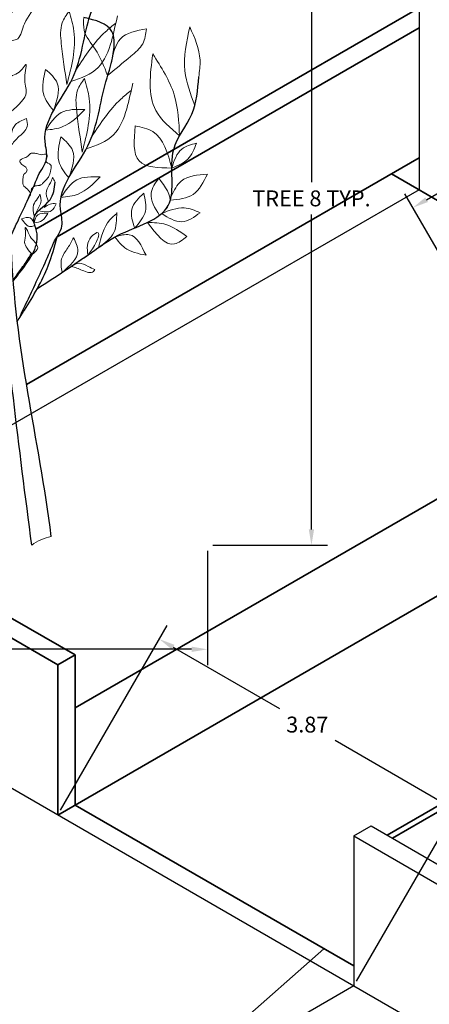
# Model space of a CAD drawing. Units: metres. Extents: x 12735 to 25554, y 20954 to 41989.
# Tile 3 of 15: x 12743.97 to 12748.61, y 20963.53 to 20974.68. Entities that reach past the tile are written whole.
import ezdxf

# ---------------------------------------------------------------- set-up
doc = ezdxf.new("R2010")
doc.units = ezdxf.units.M
doc.layers.get('Defpoints').update_dxf_attribs({"lineweight": 13})
for name, color, linetype, lineweight in [('A-ANNO-DIMS', 2, 'Continuous', 18), ('A-ELEV', 7, 'Continuous', 35), ('C-SITE', 8, 'Continuous', 25), ('TREES', 72, 'Continuous', 18)]:
    doc.layers.add(name, color=color, linetype=linetype, lineweight=lineweight)
doc.layers.add('STEM', color=32, linetype='Continuous')
doc.styles.get("Standard").update_dxf_attribs({"font": 'arial.ttf'})
doc.dimstyles.get("Standard").update_dxf_attribs({"dimtxt": 0.18, "dimasz": 0.18, "dimexe": 0.18, "dimexo": 0.0625, "dimgap": 0.09, "dimtad": 0, "dimtih": 1, "dimtoh": 1, "dimdec": 4, "dimzin": 0, "dimdsep": 46, "dimtxsty": 'Standard', "dimcen": 0.09, "dimadec": 0, "dimazin": 0, "dimtfac": 1, "dimtdec": 4, "dimtofl": 0, "dimtmove": 0, "dimatfit": 3, "dimfxl": 1, "dimtolj": 1, "dimtzin": 0, "dimarcsym": 0})

# ---------------------------------------------------------------- blocks, each defined once
blk = doc.blocks.new('TREES')
blk.add_line((12743.7, 20972.648), (12743.7, 20972.648))
at = {"layer": 'STEM'}
for points, knots in [([(12743.791, 20972.546), (12743.793, 20972.564), (12743.795, 20972.582), (12743.797, 20972.6), (12743.801, 20972.637), (12743.806, 20972.674), (12743.81, 20972.711), (12743.845, 20973.018), (12743.938, 20973.826), (12743.743, 20974.806), (12743.607, 20975.634), (12743.413, 20975.893), (12743.333, 20975.999)], [-0.164913, -0.164913, -0.164913, -0.164913, -0.110972, -0.110972, -0.110972, 0, 0, 0, 0.920963, 2.426088, 2.990404, 3.384799, 3.384799, 3.384799, 3.384799]), ([(12743.7, 20972.648), (12743.691, 20972.807), (12743.671, 20973.194), (12743.257, 20973.699), (12743.111, 20974.379), (12743.038, 20974.998), (12742.993, 20975.377), (12742.974, 20975.54)], [0, 0, 0, 0, 0.469346, 1.137622, 1.869488, 2.521439, 3.013071, 3.013071, 3.013071, 3.013071]), ([(12743.874, 20972.227), (12743.898, 20972.277), (12743.921, 20972.328), (12743.945, 20972.378), (12744.022, 20972.541), (12744.105, 20972.717), (12744.205, 20972.963), (12744.312, 20973.088), (12744.183, 20973.501), (12744.667, 20973.973), (12744.707, 20974.64), (12744.896, 20975.012), (12744.823, 20975.434), (12744.85, 20975.23), (12744.867, 20975.1)], [-0.166951, -0.166951, -0.166951, -0.166951, 0, 0, 0, 0.539768, 0.582066, 0.798222, 0.98781, 1.7696, 2.524754, 2.899414, 3.105113, 3.460848, 3.460848, 3.460848, 3.460848]), ([(12743.728, 20972.218), (12743.63, 20972.372), (12743.383, 20972.76), (12742.753, 20973.07), (12742.291, 20973.419), (12741.984, 20973.759), (12741.959, 20974.098), (12741.675, 20974.346), (12741.563, 20974.543), (12741.494, 20974.663)], [0, 0, 0, 0, 0.542161, 1.359078, 2.03444, 2.290187, 2.703676, 2.968549, 3.382864, 3.382864, 3.382864, 3.382864]), ([(12743.967, 20971.294), (12743.987, 20971.335), (12744.006, 20971.376), (12744.026, 20971.417), (12744.057, 20971.483), (12744.088, 20971.549), (12744.119, 20971.615), (12744.196, 20971.778), (12744.279, 20971.954), (12744.378, 20972.2), (12744.486, 20972.325), (12744.357, 20972.738), (12744.836, 20973.215), (12744.895, 20973.862), (12745.051, 20974.269), (12745.045, 20974.62), (12744.834, 20974.67), (12744.7, 20974.701)], [-0.355099, -0.355099, -0.355099, -0.355099, -0.218492, -0.218492, -0.218492, 0, 0, 0, 0.539768, 0.582066, 0.798222, 0.98781, 1.7696, 2.524754, 2.899414, 3.105113, 3.460848, 3.460848, 3.460848, 3.460848]), ([(12744.175, 20971.633), (12744.383, 20971.767), (12744.692, 20971.967), (12745.149, 20972.305), (12745.828, 20972.463), (12745.606, 20973.185), (12745.967, 20973.583), (12745.99, 20973.882), (12746.002, 20974.029)], [0, 0, 0, 0, 0.736164, 1.094646, 1.754618, 2.392389, 2.840214, 3.27091, 3.27091, 3.27091, 3.27091]), ([(12743.381, 20973.588), (12743.52, 20973.4), (12743.728, 20973.118), (12743.725, 20972.776), (12743.724, 20972.661), (12743.724, 20972.661), (12743.724, 20972.661), (12743.724, 20972.661), (12743.724, 20972.65), (12743.724, 20972.639), (12743.724, 20972.627)], [0, 0, 0, 0, 0.673099, 1.009429, 1.009429, 1.009429, 1.009429, 1.009429, 1.009429, 1.043412, 1.043412, 1.043412, 1.043412]), ([(12743.814, 20972.505), (12743.817, 20972.531), (12743.819, 20972.556), (12743.822, 20972.581), (12743.827, 20972.63), (12743.832, 20972.679), (12743.838, 20972.727), (12743.847, 20972.813), (12743.865, 20972.982), (12743.864, 20973.152), (12743.864, 20973.236)], [-0.2227932, -0.2227932, -0.2227932, -0.2227932, -0.1464713, -0.1464713, -0.1464713, 0, 0, 0, 0.2578951, 0.5103882, 0.5103882, 0.5103882, 0.5103882]), ([(12743.902, 20971.717), (12743.93, 20971.754), (12743.959, 20971.791), (12743.988, 20971.829), (12743.988, 20971.829), (12743.988, 20971.829), (12743.988, 20971.829), (12744.096, 20971.973), (12744.236, 20972.16), (12744.082, 20972.476), (12744.347, 20972.598), (12744.368, 20972.766), (12744.376, 20972.837)], [-0.129757, -0.129757, -0.129757, -0.129757, 0, 0, 0, 0, 0, 0, 0.485118, 0.62751, 0.913144, 1.120766, 1.120766, 1.120766, 1.120766]), ([(12744.111, 20968.725), (12743.967, 20969.837), (12743.799, 20971.142), (12743.712, 20972.453), (12743.7, 20972.648)], [0, 0, 0, 0, 3.359203, 3.944548, 3.944548, 3.944548, 3.944548]), ([(12744.332, 20968.825), (12744.189, 20969.936), (12743.871, 20971.161), (12743.872, 20972.51), (12743.7, 20972.648)], [0, 0, 0, 0, 3.359203, 3.972384, 3.972384, 3.972384, 3.972384]), ([(12743.597, 20972.418), (12743.533, 20972.41), (12743.292, 20972.379), (12742.889, 20972.351), (12742.364, 20972.241), (12741.803, 20972.489), (12741.157, 20972.302), (12740.698, 20972.258), (12740.474, 20972.237)], [0, 0, 0, 0, 0.193148, 0.727923, 1.218416, 1.762371, 2.471743, 3.152626, 3.152626, 3.152626, 3.152626]), ([(12743.181, 20972.372), (12743.296, 20972.37), (12743.441, 20972.368), (12743.583, 20972.39), (12743.613, 20972.395)], [0, 0, 0, 0, 0.3435042, 0.4329772, 0.4329772, 0.4329772, 0.4329772]), ([(12743.948, 20971.264), (12743.975, 20971.305), (12744.002, 20971.345), (12744.029, 20971.386), (12744.029, 20971.386), (12744.029, 20971.386), (12744.029, 20971.386), (12744.129, 20971.55), (12744.289, 20971.812), (12744.368, 20972.107), (12744.398, 20972.218)], [-0.148605, -0.148605, -0.148605, -0.148605, 0, 0, 0, 0, 0, 0, 0.572176, 0.914425, 0.914425, 0.914425, 0.914425]), ([(12743.901, 20971.729), (12743.929, 20971.768), (12743.958, 20971.808), (12743.986, 20971.847), (12743.986, 20971.847), (12743.986, 20971.847), (12743.986, 20971.847), (12744.02, 20971.892), (12744.062, 20971.951), (12744.099, 20972.014), (12744.107, 20972.028)], [-0.1467707, -0.1467707, -0.1467707, -0.1467707, 0, 0, 0, 0, 0, 0, 0.1684242, 0.2179474, 0.2179474, 0.2179474, 0.2179474]), ([(12743.81, 20971.258), (12743.646, 20971.316), (12743.283, 20971.443), (12742.486, 20971.453), (12741.888, 20971.61), (12741.494, 20971.714)], [0, 0, 0, 0, 0.519056, 1.146346, 2.366016, 2.366016, 2.366016, 2.366016])]:
    blk.add_open_spline(points, degree=3, knots=knots, dxfattribs=at)
blk.add_open_spline([(12744.644, 20971.941), (12744.672, 20971.961), (12744.701, 20971.98), (12744.73, 20972)], degree=3, dxfattribs=at)
at = {"layer": 'TREES'}
for points, knots in [([(12743.584, 20975.586), (12743.37, 20975.718), (12743.075, 20975.9), (12743.022, 20976.725), (12743.333, 20976.097), (12743.574, 20975.612)], [0, 0, 0, 0, 0.724771, 1.002271, 1.932196, 1.932196, 1.932196, 1.932196]), ([(12743.021, 20975.14), (12743.019, 20975.277), (12743.016, 20975.483), (12742.921, 20975.662), (12742.889, 20975.721)], [0, 0, 0, 0, 0.4023849, 0.6031293, 0.6031293, 0.6031293, 0.6031293]), ([(12743.021, 20975.14), (12742.985, 20975.224), (12742.928, 20975.356), (12742.766, 20975.539), (12742.854, 20975.638), (12742.901, 20975.69)], [0, 0, 0, 0, 0.2845416, 0.4465287, 0.6279758, 0.6279758, 0.6279758, 0.6279758]), ([(12743.718, 20974.979), (12743.671, 20975.164), (12743.598, 20975.454), (12743.323, 20975.534), (12743.223, 20975.563)], [0, 0, 0, 0, 0.519429, 0.8155501, 0.8155501, 0.8155501, 0.8155501]), ([(12743.223, 20975.563), (12743.266, 20975.448), (12743.36, 20975.195), (12743.592, 20975.055), (12743.718, 20974.979)], [0, 0, 0, 0, 0.3595778, 0.7860105, 0.7860105, 0.7860105, 0.7860105]), ([(12743.737, 20974.871), (12743.729, 20975.055), (12743.718, 20975.333), (12743.914, 20975.516), (12743.981, 20975.578)], [0, 0, 0, 0, 0.5134638, 0.7779111, 0.7779111, 0.7779111, 0.7779111]), ([(12743.737, 20974.871), (12743.801, 20974.971), (12743.939, 20975.186), (12743.966, 20975.441), (12743.981, 20975.578)], [0, 0, 0, 0, 0.351068, 0.7565079, 0.7565079, 0.7565079, 0.7565079]), ([(12741.648, 20974.411), (12741.519, 20974.547), (12741.281, 20974.798), (12741.642, 20974.995), (12741.673, 20975.511), (12741.684, 20975.149), (12741.787, 20975.033), (12741.768, 20974.824), (12741.781, 20974.575), (12741.641, 20974.411), (12741.569, 20974.326)], [0, 0, 0, 0, 0.446457, 0.821839, 1.096823, 1.294203, 1.491123, 1.594729, 1.894892, 2.216107, 2.216107, 2.216107, 2.216107]), ([(12743.031, 20975.058), (12743.048, 20975.139), (12743.077, 20975.281), (12743.184, 20975.377), (12743.231, 20975.418)], [0, 0, 0, 0, 0.2398723, 0.4207027, 0.4207027, 0.4207027, 0.4207027]), ([(12743.037, 20975.007), (12743.075, 20975.058), (12743.166, 20975.181), (12743.207, 20975.33), (12743.231, 20975.418)], [0, 0, 0, 0, 0.1895117, 0.457602, 0.457602, 0.457602, 0.457602]), ([(12744.796, 20974.806), (12744.757, 20974.909), (12744.688, 20975.088), (12744.514, 20975.28), (12744.523, 20975.414), (12744.526, 20975.464)], [0, 0, 0, 0, 0.3323117, 0.5782809, 0.7232611, 0.7232611, 0.7232611, 0.7232611]), ([(12744.805, 20974.813), (12744.804, 20974.918), (12744.803, 20975.076), (12744.822, 20975.37), (12744.643, 20975.427), (12744.526, 20975.464)], [0, 0, 0, 0, 0.3224266, 0.4885617, 0.8037384, 0.8037384, 0.8037384, 0.8037384]), ([(12743.07, 20974.733), (12742.98, 20974.863), (12742.848, 20975.053), (12742.433, 20975.446), (12742.649, 20974.915), (12742.651, 20974.573), (12742.961, 20974.576), (12743.034, 20974.678), (12743.071, 20974.73)], [0, 0, 0, 0, 0.54832, 0.799685, 1.166614, 1.565159, 1.742127, 1.925713, 1.925713, 1.925713, 1.925713]), ([(12744.796, 20974.806), (12744.882, 20974.878), (12745.017, 20974.992), (12745.211, 20975.15), (12745.228, 20975.277), (12745.236, 20975.337)], [0, 0, 0, 0, 0.3416822, 0.5370609, 0.7122352, 0.7122352, 0.7122352, 0.7122352]), ([(12744.839, 20974.951), (12744.859, 20975.055), (12744.903, 20975.272), (12745.122, 20975.315), (12745.236, 20975.337)], [0, 0, 0, 0, 0.2913456, 0.6064398, 0.6064398, 0.6064398, 0.6064398]), ([(12743.814, 20974.4), (12743.798, 20974.494), (12743.764, 20974.693), (12744.115, 20975.006), (12744.156, 20974.79), (12744.01, 20974.677), (12743.989, 20974.434), (12743.864, 20974.438), (12743.809, 20974.439)], [0, 0, 0, 0, 0.311146, 0.650746, 0.669061, 0.940573, 1.125337, 1.270427, 1.270427, 1.270427, 1.270427]), ([(12743.191, 20974.047), (12743.14, 20974.139), (12743.026, 20974.346), (12743.367, 20974.877), (12743.354, 20974.597), (12743.309, 20974.413), (12743.358, 20974.125), (12743.218, 20974.059), (12743.191, 20974.047)], [0, 0, 0, 0, 0.337622, 0.758697, 0.837919, 1.040495, 1.406258, 1.489574, 1.489574, 1.489574, 1.489574]), ([(12742.028, 20973.754), (12742.003, 20973.912), (12741.953, 20974.218), (12742.174, 20974.414), (12742.283, 20974.81), (12742.258, 20974.48), (12742.304, 20974.323), (12742.246, 20974.069), (12742.227, 20973.932), (12742.006, 20973.671), (12742.066, 20973.72), (12742.075, 20973.727)], [0, 0, 0, 0, 0.436736, 0.842969, 1.012738, 1.21393, 1.403734, 1.613178, 1.897283, 2.067562, 2.097274, 2.097274, 2.097274, 2.097274]), ([(12744.509, 20973.941), (12744.486, 20974.093), (12744.451, 20974.322), (12744.425, 20974.623), (12744.504, 20974.731), (12744.534, 20974.773)], [0, 0, 0, 0, 0.4681587, 0.7056034, 0.8580265, 0.8580265, 0.8580265, 0.8580265]), ([(12744.534, 20974.773), (12744.556, 20974.698), (12744.634, 20974.425), (12744.562, 20974.144), (12744.509, 20973.941)], [0, 0, 0, 0, 0.2327329, 0.8431329, 0.8431329, 0.8431329, 0.8431329]), ([(12744.554, 20973.975), (12744.669, 20974.016), (12744.893, 20974.094), (12745.019, 20974.421), (12745.06, 20974.624), (12745.08, 20974.72)], [0, 0, 0, 0, 0.348929, 0.678298, 0.9763146, 0.9763146, 0.9763146, 0.9763146]), ([(12743.835, 20974.249), (12743.789, 20974.346), (12743.724, 20974.484), (12743.556, 20974.594), (12743.468, 20974.601), (12743.424, 20974.604)], [0, 0, 0, 0, 0.3158223, 0.4463774, 0.5774617, 0.5774617, 0.5774617, 0.5774617]), ([(12743.424, 20974.604), (12743.442, 20974.527), (12743.487, 20974.324), (12743.715, 20974.191), (12743.841, 20974.206), (12743.841, 20974.206)], [0, 0, 0, 0, 0.2361186, 0.6165307, 0.6167763, 0.6167763, 0.6167763, 0.6167763]), ([(12744.618, 20974.118), (12744.717, 20974.268), (12744.844, 20974.462), (12745.022, 20974.606), (12745.062, 20974.638)], [0, 0, 0, 0, 0.5333846, 0.686651, 0.686651, 0.686651, 0.686651]), ([(12744.97, 20974.043), (12744.931, 20974.146), (12744.862, 20974.325), (12744.688, 20974.517), (12744.697, 20974.651), (12744.7, 20974.701)], [0, 0, 0, 0, 0.3323117, 0.5782809, 0.7232611, 0.7232611, 0.7232611, 0.7232611]), ([(12745.957, 20973.706), (12745.908, 20973.835), (12745.798, 20974.123), (12745.864, 20974.427), (12745.9, 20974.594)], [0, 0, 0, 0, 0.4051126, 0.906838, 0.906838, 0.906838, 0.906838]), ([(12745.9, 20974.594), (12745.955, 20974.471), (12746.037, 20974.287), (12746.01, 20974.092), (12746.002, 20974.029)], [0, 0, 0, 0, 0.3943838, 0.5836156, 0.5836156, 0.5836156, 0.5836156]), ([(12744.97, 20974.043), (12745.056, 20974.115), (12745.191, 20974.229), (12745.385, 20974.387), (12745.402, 20974.514), (12745.41, 20974.574)], [0, 0, 0, 0, 0.3416822, 0.5370609, 0.7122352, 0.7122352, 0.7122352, 0.7122352]), ([(12745.013, 20974.188), (12745.033, 20974.292), (12745.077, 20974.509), (12745.296, 20974.552), (12745.41, 20974.574)], [0, 0, 0, 0, 0.2913456, 0.6064398, 0.6064398, 0.6064398, 0.6064398]), ([(12743.128, 20974.182), (12743.019, 20974.275), (12742.841, 20974.427), (12742.65, 20974.313), (12742.577, 20974.27)], [0, 0, 0, 0, 0.3785086, 0.6144536, 0.6144536, 0.6144536, 0.6144536]), ([(12742.577, 20974.27), (12742.635, 20974.174), (12742.755, 20973.977), (12743.187, 20974.003), (12743.173, 20974.131), (12743.172, 20974.137)], [0, 0, 0, 0, 0.3386751, 0.6999446, 0.7185805, 0.7185805, 0.7185805, 0.7185805]), ([(12745.785, 20973.361), (12745.68, 20973.449), (12745.404, 20973.684), (12745.451, 20974.057), (12745.481, 20974.288)], [0, 0, 0, 0, 0.391493, 1.034106, 1.034106, 1.034106, 1.034106]), ([(12745.481, 20974.288), (12745.577, 20974.138), (12745.76, 20973.855), (12745.777, 20973.519), (12745.785, 20973.361)], [0, 0, 0, 0, 0.5245256, 0.9915723, 0.9915723, 0.9915723, 0.9915723]), ([(12741.943, 20974.016), (12741.835, 20974.13), (12741.594, 20974.382), (12741.272, 20973.991), (12740.687, 20974.27), (12741.289, 20973.836), (12741.63, 20973.742), (12741.878, 20973.799), (12742.016, 20973.831)], [0, 0, 0, 0, 0.397812, 0.88569, 1.156328, 1.66735, 1.991498, 2.394837, 2.394837, 2.394837, 2.394837]), ([(12743.879, 20973.555), (12743.816, 20973.752), (12743.731, 20974.021), (12743.982, 20974.067), (12744.068, 20974.224), (12744.006, 20973.984), (12744.093, 20973.824), (12743.961, 20973.709), (12743.879, 20973.638)], [0, 0, 0, 0, 0.469961, 0.638827, 0.705595, 0.853148, 1.022788, 1.296962, 1.296962, 1.296962, 1.296962]), ([(12744.356, 20973.647), (12744.309, 20973.708), (12744.202, 20973.846), (12744.245, 20974.018), (12744.268, 20974.113)], [0, 0, 0, 0, 0.2209277, 0.4981889, 0.4981889, 0.4981889, 0.4981889]), ([(12744.268, 20974.113), (12744.323, 20974.065), (12744.46, 20973.94), (12744.395, 20973.758), (12744.356, 20973.647)], [0, 0, 0, 0, 0.203616, 0.5174389, 0.5174389, 0.5174389, 0.5174389]), ([(12742.389, 20973.356), (12742.341, 20973.437), (12742.234, 20973.617), (12742.458, 20973.799), (12742.48, 20973.946), (12742.486, 20973.991)], [0, 0, 0, 0, 0.251735, 0.5591808, 0.6938707, 0.6938707, 0.6938707, 0.6938707]), ([(12742.486, 20973.991), (12742.542, 20973.959), (12742.68, 20973.88), (12742.598, 20973.572), (12742.464, 20973.433), (12742.389, 20973.356)], [0, 0, 0, 0, 0.1746142, 0.4385715, 0.7703441, 0.7703441, 0.7703441, 0.7703441]), ([(12743.381, 20973.588), (12743.369, 20973.67), (12743.344, 20973.833), (12743.453, 20973.958), (12743.508, 20974.02)], [0, 0, 0, 0, 0.2360196, 0.4713289, 0.4713289, 0.4713289, 0.4713289]), ([(12743.381, 20973.588), (12743.434, 20973.649), (12743.541, 20973.774), (12743.519, 20973.937), (12743.508, 20974.02)], [0, 0, 0, 0, 0.2309694, 0.4699481, 0.4699481, 0.4699481, 0.4699481]), ([(12744.683, 20973.178), (12744.66, 20973.33), (12744.625, 20973.559), (12744.599, 20973.86), (12744.677, 20973.968), (12744.708, 20974.01)], [0, 0, 0, 0, 0.4681587, 0.7056034, 0.8580265, 0.8580265, 0.8580265, 0.8580265]), ([(12744.708, 20974.01), (12744.73, 20973.935), (12744.807, 20973.662), (12744.735, 20973.381), (12744.683, 20973.178)], [0, 0, 0, 0, 0.2327329, 0.8431329, 0.8431329, 0.8431329, 0.8431329]), ([(12744.728, 20973.213), (12744.843, 20973.253), (12745.067, 20973.331), (12745.193, 20973.658), (12745.234, 20973.861), (12745.254, 20973.957)], [0, 0, 0, 0, 0.348929, 0.678298, 0.9763146, 0.9763146, 0.9763146, 0.9763146]), ([(12743.851, 20973.09), (12743.747, 20973.196), (12743.578, 20973.368), (12743.647, 20973.644), (12743.671, 20973.769), (12743.679, 20973.81)], [0, 0, 0, 0, 0.4076044, 0.6640272, 0.7921335, 0.7921335, 0.7921335, 0.7921335]), ([(12743.679, 20973.81), (12743.708, 20973.778), (12743.776, 20973.703), (12743.798, 20973.443), (12743.829, 20973.238), (12743.851, 20973.09)], [0, 0, 0, 0, 0.125659, 0.2981213, 0.7527794, 0.7527794, 0.7527794, 0.7527794]), ([(12744.792, 20973.355), (12744.891, 20973.505), (12745.018, 20973.699), (12745.196, 20973.843), (12745.236, 20973.876)], [0, 0, 0, 0, 0.5333846, 0.686651, 0.686651, 0.686651, 0.686651]), ([(12743.364, 20973.617), (12743.288, 20973.661), (12743.124, 20973.754), (12742.939, 20973.715), (12742.84, 20973.694)], [0, 0, 0, 0, 0.2535199, 0.5460217, 0.5460217, 0.5460217, 0.5460217]), ([(12742.221, 20973.506), (12741.989, 20973.602), (12741.674, 20973.731), (12741.536, 20973.471), (12741.5, 20973.404)], [0, 0, 0, 0, 0.6060397, 0.8197481, 0.8197481, 0.8197481, 0.8197481]), ([(12743.253, 20972.784), (12743.147, 20972.854), (12742.919, 20973.005), (12742.8, 20973.728), (12742.973, 20973.491), (12743.022, 20973.422)], [0, 0, 0, 0, 0.420416, 0.90702, 1.103207, 1.103207, 1.103207, 1.103207]), ([(12742.84, 20973.694), (12742.956, 20973.634), (12743.128, 20973.545), (12743.306, 20973.6), (12743.364, 20973.617)], [0, 0, 0, 0, 0.369417, 0.546183, 0.546183, 0.546183, 0.546183]), ([(12744.268, 20973.425), (12744.32, 20973.505), (12744.424, 20973.666), (12744.615, 20973.662), (12744.711, 20973.66)], [0, 0, 0, 0, 0.2669279, 0.5349854, 0.5349854, 0.5349854, 0.5349854]), ([(12744.268, 20973.425), (12744.336, 20973.433), (12744.51, 20973.454), (12744.635, 20973.582), (12744.711, 20973.66)], [0, 0, 0, 0, 0.1990667, 0.5143408, 0.5143408, 0.5143408, 0.5143408]), ([(12741.493, 20973.429), (12741.634, 20973.396), (12741.906, 20973.333), (12742.16, 20973.449), (12742.283, 20973.505)], [0, 0, 0, 0, 0.420024, 0.8136231, 0.8136231, 0.8136231, 0.8136231]), ([(12743.864, 20973.236), (12743.891, 20973.272), (12743.952, 20973.35), (12744.077, 20973.438), (12744.058, 20973.527), (12744.051, 20973.558)], [0, 0, 0, 0, 0.1377377, 0.3031534, 0.3935537, 0.3935537, 0.3935537, 0.3935537]), ([(12743.866, 20973.267), (12743.872, 20973.352), (12743.881, 20973.49), (12744.004, 20973.539), (12744.051, 20973.558)], [0, 0, 0, 0, 0.2295676, 0.3730638, 0.3730638, 0.3730638, 0.3730638]), ([(12743.022, 20973.422), (12743.059, 20973.426), (12743.334, 20973.456), (12743.256, 20972.956), (12743.349, 20972.723), (12743.36, 20972.696)], [0, 0, 0, 0, 0.1039343, 0.7792863, 0.8705393, 0.8705393, 0.8705393, 0.8705393]), ([(12745.697, 20972.996), (12745.547, 20972.999), (12745.238, 20973.004), (12745.268, 20973.314), (12745.283, 20973.473)], [0, 0, 0, 0, 0.3799868, 0.779071, 0.779071, 0.779071, 0.779071]), ([(12745.283, 20973.473), (12745.354, 20973.458), (12745.585, 20973.409), (12745.651, 20973.165), (12745.697, 20972.996)], [0, 0, 0, 0, 0.2074949, 0.6743984, 0.6743984, 0.6743984, 0.6743984]), ([(12741.595, 20972.406), (12741.523, 20972.496), (12741.318, 20972.752), (12741.336, 20973.087), (12741.348, 20973.304)], [0, 0, 0, 0, 0.3390919, 0.9589007, 0.9589007, 0.9589007, 0.9589007]), ([(12741.348, 20973.304), (12741.406, 20973.227), (12741.6, 20972.969), (12741.591, 20972.637), (12741.585, 20972.405)], [0, 0, 0, 0, 0.2865181, 0.9509807, 0.9509807, 0.9509807, 0.9509807]), ([(12743.621, 20973.151), (12743.561, 20973.233), (12743.473, 20973.354), (12743.333, 20973.334), (12743.288, 20973.327)], [0, 0, 0, 0, 0.2726158, 0.4022356, 0.4022356, 0.4022356, 0.4022356]), ([(12743.288, 20973.327), (12743.325, 20973.265), (12743.399, 20973.138), (12743.546, 20973.147), (12743.621, 20973.151)], [0, 0, 0, 0, 0.199886, 0.4070645, 0.4070645, 0.4070645, 0.4070645]), ([(12744.53, 20972.884), (12744.482, 20972.945), (12744.376, 20973.084), (12744.419, 20973.255), (12744.442, 20973.351)], [0, 0, 0, 0, 0.2209277, 0.4981889, 0.4981889, 0.4981889, 0.4981889]), ([(12744.442, 20973.351), (12744.496, 20973.302), (12744.634, 20973.177), (12744.569, 20972.995), (12744.53, 20972.884)], [0, 0, 0, 0, 0.203616, 0.5174389, 0.5174389, 0.5174389, 0.5174389]), ([(12745.697, 20972.996), (12745.724, 20973.08), (12745.77, 20973.226), (12745.915, 20973.262), (12745.976, 20973.277)], [0, 0, 0, 0, 0.2439478, 0.4222058, 0.4222058, 0.4222058, 0.4222058]), ([(12745.697, 20972.996), (12745.764, 20973.024), (12745.897, 20973.078), (12745.95, 20973.211), (12745.976, 20973.277)], [0, 0, 0, 0, 0.2073861, 0.4117039, 0.4117039, 0.4117039, 0.4117039]), ([(12744.074, 20972.655), (12744.086, 20972.673), (12744.124, 20972.731), (12743.998, 20972.782), (12744.014, 20972.867), (12744.011, 20972.925), (12744.052, 20972.944), (12744.07, 20973.015), (12743.988, 20973.027), (12743.97, 20973.091), (12744.03, 20973.11), (12744.072, 20973.132), (12744.097, 20973.169), (12744.133, 20973.163), (12744.172, 20973.164), (12744.216, 20973.136), (12744.296, 20973.17), (12744.282, 20973.105), (12744.259, 20973.057), (12744.341, 20973.048), (12744.328, 20972.986), (12744.32, 20972.935), (12744.299, 20972.884), (12744.258, 20972.852), (12744.236, 20972.821), (12744.215, 20972.805), (12744.179, 20972.793), (12744.139, 20972.807), (12744.095, 20972.746), (12744.111, 20972.739), (12744.111, 20972.739)], [0, 0, 0, 0, 0.055886, 0.185472, 0.25227, 0.305988, 0.338368, 0.378405, 0.48523, 0.4997, 0.565031, 0.618654, 0.656012, 0.680602, 0.71942, 0.77395, 0.836088, 0.890088, 0.913694, 0.979696, 1.032481, 1.0683, 1.142133, 1.186825, 1.224162, 1.25438, 1.26551, 1.333296, 1.383591, 1.385324, 1.385324, 1.385324, 1.385324]), ([(12742.983, 20972.961), (12742.799, 20973.009), (12742.463, 20973.098), (12742.071, 20972.928), (12741.893, 20972.798), (12741.839, 20972.759)], [0, 0, 0, 0, 0.553894, 1.01265, 1.215779, 1.215779, 1.215779, 1.215779]), ([(12743.669, 20972.977), (12743.606, 20973.025), (12743.504, 20973.102), (12743.398, 20973.043), (12743.358, 20973.021)], [0, 0, 0, 0, 0.2119595, 0.340544, 0.340544, 0.340544, 0.340544]), ([(12741.839, 20972.759), (12741.949, 20972.7), (12742.323, 20972.501), (12742.684, 20972.786), (12742.939, 20972.987)], [0, 0, 0, 0, 0.355589, 1.206871, 1.206871, 1.206871, 1.206871]), ([(12743.358, 20973.021), (12743.426, 20972.983), (12743.527, 20972.926), (12743.633, 20972.964), (12743.669, 20972.977)], [0, 0, 0, 0, 0.2166399, 0.3265492, 0.3265492, 0.3265492, 0.3265492]), ([(12745.681, 20972.634), (12745.776, 20972.643), (12745.97, 20972.661), (12746.056, 20972.838), (12746.1, 20972.929)], [0, 0, 0, 0, 0.2646598, 0.5464061, 0.5464061, 0.5464061, 0.5464061]), ([(12745.691, 20972.679), (12745.723, 20972.743), (12745.803, 20972.904), (12745.989, 20972.919), (12746.1, 20972.929)], [0, 0, 0, 0, 0.2025395, 0.5100625, 0.5100625, 0.5100625, 0.5100625]), ([(12741.358, 20972.366), (12741.291, 20972.434), (12741.162, 20972.564), (12740.909, 20972.646), (12740.492, 20972.989), (12740.719, 20972.381), (12740.905, 20972.253), (12741.437, 20972.382), (12741.361, 20972.366), (12741.358, 20972.366)], [0, 0, 0, 0, 0.274554, 0.529523, 0.902439, 1.220606, 1.740632, 1.953969, 1.962894, 1.962894, 1.962894, 1.962894]), ([(12742.858, 20972.779), (12743.034, 20972.81), (12743.375, 20972.87), (12743.295, 20972.539), (12743.257, 20972.379)], [0, 0, 0, 0, 0.4156133, 0.8046117, 0.8046117, 0.8046117, 0.8046117]), ([(12744.299, 20972.615), (12744.284, 20972.657), (12744.255, 20972.734), (12744.322, 20972.816), (12744.34, 20972.869), (12744.347, 20972.89)], [0, 0, 0, 0, 0.1248577, 0.2264879, 0.2926557, 0.2926557, 0.2926557, 0.2926557]), ([(12744.442, 20972.662), (12744.494, 20972.743), (12744.598, 20972.903), (12744.789, 20972.899), (12744.885, 20972.897)], [0, 0, 0, 0, 0.2669279, 0.5349854, 0.5349854, 0.5349854, 0.5349854]), ([(12744.442, 20972.662), (12744.51, 20972.671), (12744.684, 20972.691), (12744.809, 20972.819), (12744.885, 20972.897)], [0, 0, 0, 0, 0.1990667, 0.5143408, 0.5143408, 0.5143408, 0.5143408]), ([(12745.557, 20972.46), (12745.505, 20972.545), (12745.415, 20972.69), (12745.509, 20972.826), (12745.548, 20972.882)], [0, 0, 0, 0, 0.2672291, 0.4594629, 0.4594629, 0.4594629, 0.4594629]), ([(12745.548, 20972.882), (12745.623, 20972.785), (12745.735, 20972.639), (12745.619, 20972.519), (12745.581, 20972.479)], [0, 0, 0, 0, 0.3063433, 0.4579535, 0.4579535, 0.4579535, 0.4579535]), ([(12743.257, 20972.379), (12743.071, 20972.409), (12742.794, 20972.453), (12742.842, 20972.698), (12742.858, 20972.779)], [0, 0, 0, 0, 0.4478858, 0.6692237, 0.6692237, 0.6692237, 0.6692237]), ([(12744.14, 20972.455), (12744.129, 20972.498), (12744.112, 20972.571), (12744.173, 20972.643), (12744.195, 20972.684), (12744.204, 20972.7)], [0, 0, 0, 0, 0.124617, 0.2107396, 0.2658134, 0.2658134, 0.2658134, 0.2658134]), ([(12744.14, 20972.455), (12744.155, 20972.485), (12744.181, 20972.535), (12744.225, 20972.615), (12744.212, 20972.669), (12744.204, 20972.7)], [0, 0, 0, 0, 0.1037237, 0.1704768, 0.2630686, 0.2630686, 0.2630686, 0.2630686]), ([(12745.276, 20972.317), (12745.252, 20972.391), (12745.204, 20972.544), (12745.32, 20972.655), (12745.379, 20972.712)], [0, 0, 0, 0, 0.2148949, 0.4418034, 0.4418034, 0.4418034, 0.4418034]), ([(12745.276, 20972.317), (12745.329, 20972.378), (12745.429, 20972.493), (12745.395, 20972.642), (12745.379, 20972.712)], [0, 0, 0, 0, 0.2259484, 0.4304915, 0.4304915, 0.4304915, 0.4304915]), ([(12740.645, 20972.254), (12740.532, 20972.287), (12740.33, 20972.345), (12740.37, 20972.543), (12740.387, 20972.63)], [0, 0, 0, 0, 0.300298, 0.5327787, 0.5327787, 0.5327787, 0.5327787]), ([(12740.387, 20972.63), (12740.446, 20972.602), (12740.598, 20972.53), (12740.627, 20972.359), (12740.645, 20972.254)], [0, 0, 0, 0, 0.1847401, 0.4807235, 0.4807235, 0.4807235, 0.4807235]), ([(12742.916, 20972.343), (12742.772, 20972.452), (12742.448, 20972.697), (12742.076, 20972.511), (12741.869, 20972.407)], [0, 0, 0, 0, 0.501704, 1.133573, 1.133573, 1.133573, 1.133573]), ([(12744.192, 20972.515), (12744.244, 20972.502), (12744.335, 20972.479), (12744.372, 20972.56), (12744.387, 20972.593)], [0, 0, 0, 0, 0.1401829, 0.239855, 0.239855, 0.239855, 0.239855]), ([(12744.25, 20972.55), (12744.272, 20972.566), (12744.314, 20972.595), (12744.364, 20972.594), (12744.387, 20972.593)], [0, 0, 0, 0, 0.0790636, 0.1468534, 0.1468534, 0.1468534, 0.1468534]), ([(12744.137, 20972.378), (12744.147, 20972.414), (12744.168, 20972.49), (12744.249, 20972.485), (12744.292, 20972.483)], [0, 0, 0, 0, 0.0982704, 0.2114853, 0.2114853, 0.2114853, 0.2114853]), ([(12744.137, 20972.378), (12744.171, 20972.382), (12744.241, 20972.388), (12744.274, 20972.45), (12744.292, 20972.483)], [0, 0, 0, 0, 0.0955829, 0.1975677, 0.1975677, 0.1975677, 0.1975677]), ([(12744.868, 20972.097), (12744.937, 20972.148), (12745.072, 20972.246), (12745.072, 20972.413), (12745.073, 20972.494)], [0, 0, 0, 0, 0.2403434, 0.4714363, 0.4714363, 0.4714363, 0.4714363]), ([(12744.868, 20972.097), (12744.895, 20972.212), (12744.931, 20972.363), (12745.046, 20972.458), (12745.074, 20972.481)], [0, 0, 0, 0, 0.3374321, 0.4432568, 0.4432568, 0.4432568, 0.4432568]), ([(12745.582, 20972.481), (12745.667, 20972.516), (12745.814, 20972.576), (12745.958, 20972.516), (12746.019, 20972.491)], [0, 0, 0, 0, 0.2625898, 0.453199, 0.453199, 0.453199, 0.453199]), ([(12745.582, 20972.481), (12745.658, 20972.433), (12745.808, 20972.341), (12745.95, 20972.442), (12746.019, 20972.491)], [0, 0, 0, 0, 0.2451587, 0.4783488, 0.4783488, 0.4783488, 0.4783488]), ([(12741.223, 20971.823), (12741.319, 20971.881), (12741.571, 20972.033), (12741.755, 20972.264), (12741.869, 20972.407)], [0, 0, 0, 0, 0.3340001, 0.876507, 0.876507, 0.876507, 0.876507]), ([(12741.595, 20972.406), (12741.515, 20972.319), (12741.356, 20972.147), (12741.267, 20971.93), (12741.223, 20971.823)], [0, 0, 0, 0, 0.3521388, 0.6963584, 0.6963584, 0.6963584, 0.6963584]), ([(12743.181, 20972.372), (12743.094, 20972.305), (12742.907, 20972.162), (12742.991, 20971.938), (12743.035, 20971.819)], [0, 0, 0, 0, 0.2977969, 0.6372286, 0.6372286, 0.6372286, 0.6372286]), ([(12743.035, 20971.819), (12743.147, 20971.88), (12743.383, 20972.009), (12743.25, 20972.247), (12743.181, 20972.372)], [0, 0, 0, 0, 0.3275492, 0.688496, 0.688496, 0.688496, 0.688496]), ([(12744.145, 20972.348), (12744.132, 20972.384), (12744.105, 20972.455), (12744.032, 20972.434), (12743.996, 20972.423)], [0, 0, 0, 0, 0.098996, 0.196743, 0.196743, 0.196743, 0.196743]), ([(12743.996, 20972.423), (12744.027, 20972.377), (12744.069, 20972.315), (12744.13, 20972.341), (12744.146, 20972.347)], [0, 0, 0, 0, 0.1368513, 0.185287, 0.185287, 0.185287, 0.185287]), ([(12745.422, 20972.381), (12745.493, 20972.379), (12745.657, 20972.373), (12745.791, 20972.276), (12745.866, 20972.222)], [0, 0, 0, 0, 0.2087211, 0.4811791, 0.4811791, 0.4811791, 0.4811791]), ([(12745.422, 20972.381), (12745.521, 20972.247), (12745.661, 20972.058), (12745.82, 20972.185), (12745.866, 20972.222)], [0, 0, 0, 0, 0.3912381, 0.5526272, 0.5526272, 0.5526272, 0.5526272]), ([(12740.645, 20972.254), (12740.54, 20972.264), (12740.318, 20972.286), (12740.252, 20972.07), (12740.216, 20971.955)], [0, 0, 0, 0, 0.2808571, 0.5946199, 0.5946199, 0.5946199, 0.5946199]), ([(12740.216, 20971.955), (12740.344, 20971.984), (12740.536, 20972.026), (12740.618, 20972.197), (12740.645, 20972.254)], [0, 0, 0, 0, 0.3624795, 0.5464116, 0.5464116, 0.5464116, 0.5464116]), ([(12740.757, 20972.265), (12740.712, 20972.237), (12740.573, 20972.15), (12740.673, 20971.993), (12740.741, 20971.887)], [0, 0, 0, 0, 0.1417373, 0.4445248, 0.4445248, 0.4445248, 0.4445248]), ([(12740.741, 20971.887), (12740.783, 20971.937), (12740.878, 20972.054), (12740.801, 20972.189), (12740.757, 20972.265)], [0, 0, 0, 0, 0.1798963, 0.4162104, 0.4162104, 0.4162104, 0.4162104]), ([(12742.453, 20972.29), (12742.257, 20972.189), (12741.999, 20972.056), (12742.001, 20971.792), (12742.002, 20971.729)], [0, 0, 0, 0, 0.5792647, 0.7616052, 0.7616052, 0.7616052, 0.7616052]), ([(12742.002, 20971.729), (12742.108, 20971.788), (12742.333, 20971.914), (12742.411, 20972.161), (12742.453, 20972.29)], [0, 0, 0, 0, 0.3533474, 0.7448355, 0.7448355, 0.7448355, 0.7448355]), ([(12744.116, 20972.018), (12744.075, 20972.065), (12744.007, 20972.143), (12744.05, 20972.231), (12744.028, 20972.351), (12744.072, 20972.271), (12744.09, 20972.201), (12744.221, 20972.106), (12744.146, 20972.042), (12744.116, 20972.018)], [0, 0, 0, 0, 0.1633748, 0.2727914, 0.3326965, 0.376171, 0.4524353, 0.6040881, 0.701786, 0.701786, 0.701786, 0.701786]), ([(12744.746, 20972.012), (12744.742, 20972.047), (12744.733, 20972.118), (12744.771, 20972.218), (12744.826, 20972.252), (12744.849, 20972.268)], [0, 0, 0, 0, 0.1066556, 0.2131282, 0.2966333, 0.2966333, 0.2966333, 0.2966333]), ([(12744.746, 20972.012), (12744.773, 20972.045), (12744.822, 20972.105), (12744.891, 20972.268), (12744.848, 20972.268), (12744.847, 20972.268)], [0, 0, 0, 0, 0.1585708, 0.2833525, 0.285588, 0.285588, 0.285588, 0.285588]), ([(12745.053, 20972.215), (12745.111, 20972.233), (12745.273, 20972.284), (12745.353, 20972.117), (12745.405, 20972.009)], [0, 0, 0, 0, 0.1646898, 0.4645687, 0.4645687, 0.4645687, 0.4645687]), ([(12744.455, 20971.815), (12744.445, 20971.868), (12744.427, 20971.97), (12744.523, 20972.088), (12744.564, 20972.169), (12744.585, 20972.208)], [0, 0, 0, 0, 0.1538132, 0.2966411, 0.4292928, 0.4292928, 0.4292928, 0.4292928]), ([(12744.455, 20971.815), (12744.544, 20971.891), (12744.679, 20972.008), (12744.609, 20972.157), (12744.585, 20972.208)], [0, 0, 0, 0, 0.3019229, 0.4589929, 0.4589929, 0.4589929, 0.4589929]), ([(12745.053, 20972.215), (12745.087, 20972.171), (12745.174, 20972.057), (12745.317, 20972.027), (12745.405, 20972.009)], [0, 0, 0, 0, 0.1638697, 0.4194041, 0.4194041, 0.4194041, 0.4194041]), ([(12742.652, 20971.471), (12742.63, 20971.58), (12742.585, 20971.809), (12742.714, 20972.005), (12742.781, 20972.107)], [0, 0, 0, 0, 0.3207709, 0.6721329, 0.6721329, 0.6721329, 0.6721329]), ([(12742.652, 20971.471), (12742.732, 20971.545), (12742.92, 20971.718), (12742.832, 20971.965), (12742.781, 20972.107)], [0, 0, 0, 0, 0.3028446, 0.7080533, 0.7080533, 0.7080533, 0.7080533]), ([(12744.561, 20971.885), (12744.589, 20971.902), (12744.651, 20971.938), (12744.742, 20971.883), (12744.801, 20971.859), (12744.827, 20971.849)], [0, 0, 0, 0, 0.0920276, 0.2010844, 0.2860976, 0.2860976, 0.2860976, 0.2860976]), ([(12742.314, 20971.521), (12742.225, 20971.627), (12742.039, 20971.851), (12741.746, 20971.851), (12741.593, 20971.851)], [0, 0, 0, 0, 0.3968877, 0.8302181, 0.8302181, 0.8302181, 0.8302181]), ([(12741.593, 20971.851), (12741.666, 20971.793), (12741.821, 20971.668), (12742.447, 20971.471), (12742.312, 20971.521), (12742.311, 20971.521)], [0, 0, 0, 0, 0.3696351, 0.7965164, 0.7990281, 0.7990281, 0.7990281, 0.7990281]), ([(12743.566, 20971.341), (12743.514, 20971.414), (12743.424, 20971.54), (12743.418, 20971.749), (12743.449, 20971.857), (12743.463, 20971.904)], [0, 0, 0, 0, 0.2632417, 0.4527737, 0.6011812, 0.6011812, 0.6011812, 0.6011812]), ([(12743.463, 20971.904), (12743.567, 20971.861), (12743.772, 20971.775), (12743.623, 20971.516), (12743.587, 20971.385), (12743.574, 20971.338)], [0, 0, 0, 0, 0.2799093, 0.5517077, 0.7021324, 0.7021324, 0.7021324, 0.7021324]), ([(12744.561, 20971.885), (12744.599, 20971.871), (12744.674, 20971.844), (12744.795, 20971.792), (12744.822, 20971.84), (12744.827, 20971.849)], [0, 0, 0, 0, 0.1330667, 0.2587888, 0.2884885, 0.2884885, 0.2884885, 0.2884885]), ([(12743.304, 20971.408), (12743.247, 20971.446), (12743.157, 20971.505), (12743.12, 20971.647), (12743.123, 20971.722), (12743.125, 20971.759)], [0, 0, 0, 0, 0.196607, 0.3084716, 0.4203856, 0.4203856, 0.4203856, 0.4203856]), ([(12743.125, 20971.759), (12743.154, 20971.73), (12743.251, 20971.635), (12743.282, 20971.501), (12743.304, 20971.408)], [0, 0, 0, 0, 0.1222515, 0.400195, 0.400195, 0.400195, 0.400195]), ([(12742.056, 20971.092), (12742.207, 20971.066), (12742.53, 20971.009), (12742.604, 20971.335), (12742.644, 20971.51)], [0, 0, 0, 0, 0.3982442, 0.8534889, 0.8534889, 0.8534889, 0.8534889]), ([(12742.547, 20971.484), (12742.396, 20971.478), (12742.124, 20971.467), (12742.077, 20971.207), (12742.056, 20971.092)], [0, 0, 0, 0, 0.3960722, 0.7115037, 0.7115037, 0.7115037, 0.7115037]), ([(12742.918, 20971.429), (12742.811, 20971.373), (12742.636, 20971.282), (12742.7, 20971.111), (12742.725, 20971.045)], [0, 0, 0, 0, 0.3055467, 0.4944991, 0.4944991, 0.4944991, 0.4944991]), ([(12742.725, 20971.045), (12742.787, 20971.086), (12742.922, 20971.175), (12742.92, 20971.34), (12742.918, 20971.429)], [0, 0, 0, 0, 0.2088213, 0.4571427, 0.4571427, 0.4571427, 0.4571427]), ([(12743.381, 20971.391), (12743.311, 20971.354), (12743.137, 20971.26), (12743.15, 20971.056), (12743.158, 20970.935)], [0, 0, 0, 0, 0.2232821, 0.551466, 0.551466, 0.551466, 0.551466]), ([(12743.158, 20970.935), (12743.238, 20970.974), (12743.421, 20971.065), (12743.396, 20971.274), (12743.381, 20971.391)], [0, 0, 0, 0, 0.2445355, 0.5611675, 0.5611675, 0.5611675, 0.5611675]), ([(12743.743, 20971.282), (12743.611, 20971.245), (12743.396, 20971.185), (12743.421, 20970.978), (12743.431, 20970.898)], [0, 0, 0, 0, 0.3473993, 0.565418, 0.565418, 0.565418, 0.565418]), ([(12743.431, 20970.898), (12743.517, 20970.939), (12743.683, 20971.018), (12743.723, 20971.196), (12743.743, 20971.282)], [0, 0, 0, 0, 0.2699816, 0.5191769, 0.5191769, 0.5191769, 0.5191769])]:
    blk.add_open_spline(points, degree=3, knots=knots, dxfattribs=at)
blk.add_open_spline([(12744.347, 20972.89), (12744.357, 20972.872), (12744.367, 20972.854), (12744.376, 20972.837)], degree=3, dxfattribs=at)
blk = doc.blocks.new('*D5')
at = {"layer": 'A-ANNO-DIMS', "color": 0, "lineweight": -2, "transparency": 16777216}
for p, q in [((12746.163, 20976.581), (12747.458, 20976.581)), ((12747.278, 20976.401), (12747.278, 20972.835)), ((12747.278, 20968.905), (12747.278, 20972.471)), ((12746.163, 20968.725), (12747.458, 20968.725))]:
    blk.add_line(p, q, dxfattribs=at)
at = {"layer": 'A-ANNO-DIMS', "color": 0, "transparency": 16777216}
for points in [[(12747.248, 20976.401), (12747.308, 20976.401), (12747.278, 20976.581)], [(12747.248, 20968.905), (12747.308, 20968.905), (12747.278, 20968.725)]]:
    blk.add_solid(points, dxfattribs=at)
at = {"layer": 'Defpoints', "color": 0, "transparency": 16777216}
for p in [(12746.1, 20976.581), (12747.278, 20976.581), (12746.1, 20968.725)]:
    blk.add_point(p, dxfattribs=at)
at = {"layer": 'A-ANNO-DIMS', "color": 0, "transparency": 16777216, "insert": (12747.278, 20972.653), "char_height": 0.18, "attachment_point": 5}
blk.add_mtext('\\A1;TREE 8 TYP.', dxfattribs=at)
blk = doc.blocks.new('*D6')
at = {"layer": 'A-ANNO-DIMS', "color": 0, "lineweight": -2, "transparency": 16777216}
for p, q in [((12740.216, 20968.663), (12740.216, 20967.367)), ((12746.1, 20968.663), (12746.1, 20967.367)), ((12740.396, 20967.547), (12742.7, 20967.547)), ((12745.92, 20967.547), (12743.617, 20967.547))]:
    blk.add_line(p, q, dxfattribs=at)
at = {"layer": 'A-ANNO-DIMS', "color": 0, "transparency": 16777216}
for points in [[(12740.396, 20967.577), (12740.396, 20967.517), (12740.216, 20967.547)], [(12745.92, 20967.577), (12745.92, 20967.517), (12746.1, 20967.547)]]:
    blk.add_solid(points, dxfattribs=at)
at = {"layer": 'Defpoints', "color": 0, "transparency": 16777216}
for p in [(12740.216, 20968.725), (12746.1, 20968.725), (12746.1, 20967.547)]:
    blk.add_point(p, dxfattribs=at)
at = {"layer": 'A-ANNO-DIMS', "color": 0, "transparency": 16777216, "insert": (12743.158, 20967.547), "char_height": 0.18, "attachment_point": 5}
blk.add_mtext('\\A1;6 TYP.', dxfattribs=at)
blk = doc.blocks.new('*D9')
at = {"layer": 'A-ANNO-DIMS', "color": 0, "lineweight": -2, "transparency": 16777216}
for p, q in [((12781.004, 20970.87), (12781.004, 20953.893)), ((12737.843, 20966.671), (12737.843, 20953.893)), ((12738.023, 20954.073), (12759.026, 20954.073)), ((12780.824, 20954.073), (12759.821, 20954.073))]:
    blk.add_line(p, q, dxfattribs=at)
at = {"layer": 'A-ANNO-DIMS', "color": 0, "transparency": 16777216}
for points in [[(12738.023, 20954.103), (12738.023, 20954.043), (12737.843, 20954.073)], [(12780.824, 20954.103), (12780.824, 20954.043), (12781.004, 20954.073)]]:
    blk.add_solid(points, dxfattribs=at)
at = {"layer": 'Defpoints', "color": 0, "transparency": 16777216}
for p in [(12781.004, 20970.933), (12737.843, 20966.733), (12781.004, 20954.073)]:
    blk.add_point(p, dxfattribs=at)
at = {"layer": 'A-ANNO-DIMS', "color": 0, "transparency": 16777216, "insert": (12759.423, 20954.073), "char_height": 0.18, "attachment_point": 5}
blk.add_mtext('\\A1;43.16', dxfattribs=at)
blk = doc.blocks.new('*D11')
at = {"layer": 'A-ANNO-DIMS', "color": 0, "lineweight": -2, "transparency": 16777216}
for p, q in [((12737.811, 20966.679), (12736.603, 20964.586)), ((12736.848, 20964.652), (12745.35, 20959.743)), ((12754.481, 20954.472), (12745.98, 20959.38)), ((12755.756, 20956.319), (12754.547, 20954.226))]:
    blk.add_line(p, q, dxfattribs=at)
at = {"layer": 'A-ANNO-DIMS', "color": 0, "transparency": 16777216}
for points in [[(12736.863, 20964.678), (12736.833, 20964.626), (12736.693, 20964.742)], [(12754.496, 20954.497), (12754.466, 20954.446), (12754.637, 20954.382)]]:
    blk.add_solid(points, dxfattribs=at)
at = {"layer": 'Defpoints', "color": 0, "transparency": 16777216}
for p in [(12737.843, 20966.733), (12736.693, 20964.742), (12755.787, 20956.373)]:
    blk.add_point(p, dxfattribs=at)
at = {"layer": 'A-ANNO-DIMS', "color": 0, "transparency": 16777216, "insert": (12745.665, 20959.562), "char_height": 0.18, "attachment_point": 5}
blk.add_mtext('\\A1;20.72', dxfattribs=at)
blk = doc.blocks.new('*D21')
at = {"layer": 'A-ANNO-DIMS', "color": 0, "lineweight": -2, "transparency": 16777216}
for p, q in [((12747.361, 20976.07), (12748.57, 20978.164)), ((12748.636, 20977.918), (12751.37, 20976.339)), ((12754.734, 20974.397), (12752, 20975.976)), ((12753.771, 20972.369), (12754.98, 20974.463))]:
    blk.add_line(p, q, dxfattribs=at)
at = {"layer": 'A-ANNO-DIMS', "color": 0, "transparency": 16777216}
for points in [[(12748.651, 20977.944), (12748.621, 20977.892), (12748.48, 20978.008)], [(12754.749, 20974.423), (12754.719, 20974.371), (12754.89, 20974.307)]]:
    blk.add_solid(points, dxfattribs=at)
at = {"layer": 'Defpoints', "color": 0, "transparency": 16777216}
for p in [(12747.33, 20976.016), (12754.89, 20974.307), (12753.74, 20972.315)]:
    blk.add_point(p, dxfattribs=at)
at = {"layer": 'A-ANNO-DIMS', "color": 0, "transparency": 16777216, "insert": (12751.685, 20976.158), "char_height": 0.18, "attachment_point": 5}
blk.add_mtext('\\A1;7.402', dxfattribs=at)
blk = doc.blocks.new('*D24')
at = {"layer": 'A-ANNO-DIMS', "color": 0, "lineweight": -2, "transparency": 16777216}
for p, q in [((12744.437, 20965.724), (12745.646, 20967.818)), ((12745.712, 20967.572), (12746.916, 20966.877)), ((12748.751, 20965.817), (12747.547, 20966.513)), ((12747.789, 20963.789), (12748.997, 20965.883))]:
    blk.add_line(p, q, dxfattribs=at)
at = {"layer": 'A-ANNO-DIMS', "color": 0, "transparency": 16777216}
for points in [[(12745.727, 20967.598), (12745.697, 20967.546), (12745.556, 20967.662)], [(12748.766, 20965.843), (12748.736, 20965.791), (12748.907, 20965.727)]]:
    blk.add_solid(points, dxfattribs=at)
at = {"layer": 'Defpoints', "color": 0, "transparency": 16777216}
for p in [(12748.907, 20965.727), (12744.406, 20965.67), (12747.757, 20963.735)]:
    blk.add_point(p, dxfattribs=at)
at = {"layer": 'A-ANNO-DIMS', "color": 0, "transparency": 16777216, "insert": (12747.231, 20966.695), "char_height": 0.18, "attachment_point": 5}
blk.add_mtext('\\A1;3.87', dxfattribs=at)
blk = doc.blocks.new('*D26')
at = {"layer": 'A-ANNO-DIMS', "color": 0, "lineweight": -2, "transparency": 16777216}
for p, q in [((12752.23, 20972.16), (12751.021, 20974.253)), ((12750.955, 20974.008), (12750.005, 20973.459)), ((12748.582, 20972.638), (12749.533, 20973.186)), ((12749.545, 20970.61), (12748.337, 20972.703))]:
    blk.add_line(p, q, dxfattribs=at)
at = {"layer": 'A-ANNO-DIMS', "color": 0, "transparency": 16777216}
for points in [[(12750.94, 20974.034), (12750.97, 20973.982), (12751.111, 20974.098)], [(12748.567, 20972.664), (12748.597, 20972.612), (12748.427, 20972.548)]]:
    blk.add_solid(points, dxfattribs=at)
at = {"layer": 'Defpoints', "color": 0, "transparency": 16777216}
for p in [(12751.111, 20974.098), (12752.261, 20972.106), (12749.577, 20970.556)]:
    blk.add_point(p, dxfattribs=at)
at = {"layer": 'A-ANNO-DIMS', "color": 0, "transparency": 16777216, "insert": (12749.769, 20973.323), "char_height": 0.18, "attachment_point": 5}
blk.add_mtext('\\A1;3.1', dxfattribs=at)

msp = doc.modelspace()

# ---------------------------------------------------------------- linework, layer by layer
at = {"layer": 'A-ELEV'}
for p, q in [((12748.4969, 20974.8107), (12744.1586, 20972.306)), ((12748.4969, 20974.5847), (12744.3977, 20972.2181)), ((12748.4969, 20973.1107), (12744.0525, 20970.5448)), ((12750.937, 20971.3411), (12748.1844, 20972.9304)), ((12749.5766, 20969.7557), (12744.6014, 20966.8833)), ((12744.4057, 20965.6703), (12750.5292, 20969.2057)), ((12743.6488, 20968.0333), (12744.6014, 20967.4833)), ((12743.4531, 20967.9203), (12744.4057, 20967.3703)), ((12752.5644, 20968.0001), (12748.1353, 20965.443)), ((12752.5644, 20967.9307), (12748.1954, 20965.4083)), ((12744.6014, 20967.4833), (12744.4057, 20967.3703)), ((12744.6014, 20967.4833), (12744.6014, 20965.7833)), ((12744.4057, 20967.3703), (12744.4057, 20965.6703)), ((12744.6014, 20965.7833), (12747.7573, 20963.9612))]:
    msp.add_line(p, q, dxfattribs=at)
at = {"layer": 'C-SITE'}
for p, q in [((12748.4969, 20975.3424), (12748.4969, 20972.75)), ((12748.4969, 20972.75), (12741.7923, 20968.8791)), ((12757.9519, 20957.8494), (12740.0077, 20968.2095)), ((12747.7573, 20965.4352), (12747.953, 20965.5482)), ((12747.953, 20965.5482), (12757.9519, 20959.7754)), ((12747.7573, 20965.4352), (12757.9519, 20959.5494)), ((12747.7573, 20965.4352), (12747.7573, 20963.7352)), ((12747.4196, 20964.1562), (12745.3965, 20962.3722)), ((12747.7573, 20963.7352), (12745.3965, 20962.3722))]:
    msp.add_line(p, q, dxfattribs=at)
at = {"layer": 'TREES'}
msp.add_arc((12744.4298, 20968.3092), 0.5245, 100.74269, 127.48848, dxfattribs=at)

# ---------------------------------------------------------------- block references
msp.add_blockref('TREES', (0, 0), dxfattribs=at)

# ---------------------------------------------------------------- dimensions: what is measured, and where the dimension line sits
at = {"layer": 'A-ANNO-DIMS'}
for base, p1, p2, angle, override, picture, middle in [((12754.8902, 20974.307), (12747.3297, 20976.0163), (12753.7402, 20972.3152), 330, {"dimdec": 3, "dimlfac": 1, "dimrnd": 0, "dimzin": 0, "dimdsep": 46, "dimlunit": 2}, '*D21', (12751.6849, 20976.1576)), ((12751.1113, 20974.0976), (12749.5766, 20970.5557), (12752.2613, 20972.1057), 30, {"dimdec": 1, "dimlfac": 1, "dimrnd": 0, "dimzin": 0, "dimdsep": 46, "dimlunit": 2}, '*D26', (12749.7689, 20973.3226)), ((12748.9073, 20965.7271), (12744.4057, 20965.6703), (12747.7573, 20963.7352), 330, {"dimdec": 2, "dimlfac": 1, "dimrnd": 0, "dimzin": 0, "dimdsep": 46, "dimlunit": 2}, '*D24', (12747.2315, 20966.6946)), ((12736.6926, 20964.7416), (12755.7869, 20956.3734), (12737.8426, 20966.7335), 150, {"dimdec": 2, "dimlfac": 1, "dimrnd": 0, "dimzin": 0, "dimdsep": 46, "dimlunit": 2}, '*D11', (12745.6647, 20959.5616))]:
    dim = msp.add_linear_dim(base=base, p1=p1, p2=p2, angle=angle, dimstyle='Standard', override=override, dxfattribs=at)
    dim.commit()
    dim.dimension.update_dxf_attribs({"geometry": picture, "text_midpoint": middle})
dim = msp.add_linear_dim(base=(12747.2785, 20976.5808), p1=(12746.1001, 20968.7254), p2=(12746.1001, 20976.5808), angle=90, text='TREE <> TYP.', dimstyle='Standard', override={"dimdec": 0, "dimlfac": 1, "dimrnd": 0, "dimzin": 0, "dimdsep": 46, "dimlunit": 2}, dxfattribs=at)
dim.commit()
dim.dimension.update_dxf_attribs({"geometry": '*D5', "text_midpoint": (12747.2785, 20972.6531)})
dim = msp.add_linear_dim(base=(12781.0041, 20954.0734), p1=(12737.8426, 20966.7335), p2=(12781.0041, 20970.9326), dimstyle='Standard', override={"dimdec": 2, "dimlfac": 1, "dimrnd": 0, "dimzin": 0, "dimdsep": 46, "dimlunit": 2}, dxfattribs=at)
dim.commit()
dim.dimension.update_dxf_attribs({"geometry": '*D9', "text_midpoint": (12759.4234, 20954.0734)})
dim = msp.add_linear_dim(base=(12746.1001, 20967.5471), p1=(12740.2163, 20968.7254), p2=(12746.1001, 20968.7254), text='<> TYP.', dimstyle='Standard', override={"dimdec": 0, "dimlfac": 1, "dimrnd": 0, "dimzin": 0, "dimdsep": 46, "dimlunit": 2}, dxfattribs=at)
dim.commit()
dim.dimension.update_dxf_attribs({"geometry": '*D6', "text_midpoint": (12743.1582, 20967.5471)})

doc.saveas('drawing.dxf')
